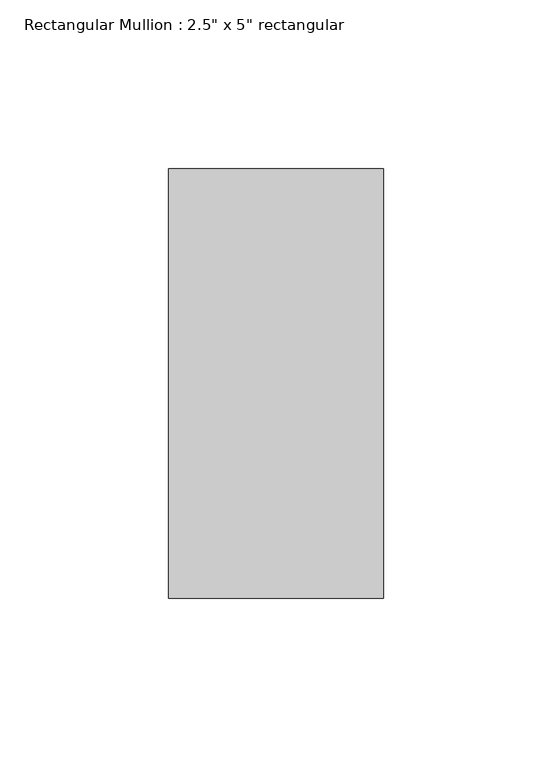
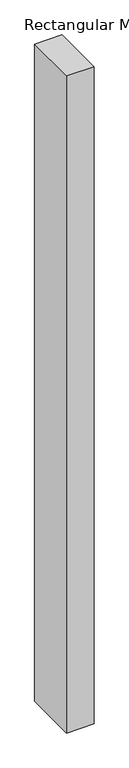
"""IFC4 building model written with IfcOpenShell, lengths in millimetres: member geometry."""

from ifc_helpers import new_model, si_unit, frame, origin, place, context, project, spatial, polyline, outline, extrude, source, transform, mapped, element, save


def member_d9503739(model_context):
    return source(origin(), model_context, "Body", "SweptSolid", [
        extrude(outline(polyline([(0.0, 63.5), (0.0, -63.5), (-63.5, -63.5), (-63.5, 63.5), (0.0, 63.5)])), frame((0.0, 0.0, -1600.2), z_axis=(0.0, 0.0, 1.0), x_axis=(1.0, 0.0, 0.0)), (0.0, 0.0, 1.0), 1600.2),
    ])


if __name__ == "__main__":
    model = new_model("IFC4")
    model_context = context("Model", 3, world=origin())
    ifc_project = project(units=[si_unit("LENGTHUNIT", "METRE", prefix="MILLI")], contexts=[model_context])
    site = spatial("IfcSite", under=ifc_project)
    building = spatial("IfcBuilding", under=site)
    placement = place(None, origin())
    member_shape = member_d9503739(model_context)
    element("IfcMember", 1, ObjectType="Rectangular Mullion : 2.5\" x 5\" rectangular", at=placement, inside=building, context=model_context, shape_type="MappedRepresentation", body=[
        mapped(member_shape, transform((0.0, 0.0, 0.0), x_axis=(1.0, 0.0, 0.0), y_axis=(0.0, 1.0, 0.0), z_axis=(0.0, 0.0, 1.0))),
    ])
    save(model, "model.ifc")

# Revit data of these elements
# Type "Rectangular Mullion : 2.5\" x 5\" rectangular"
#   built-in parameter 1007304 = 0.416667 (stored number, unit not read)
#   built-in parameter 1007301 = 0.104167 (stored number, unit not read)
#   built-in parameter 1007300 = 0.104167 (stored number, unit not read)
# Element 1 (IfcMember, "Rectangular Mullion : 2.5\" x 5\" rectangular")
#   Materials on its faces: "Aluminum"
# Materials
#   "Aluminum": class "Metal", colour RGB 247 247 247, transparency 0, Description = "Aluminum 6061", Cost = 0
